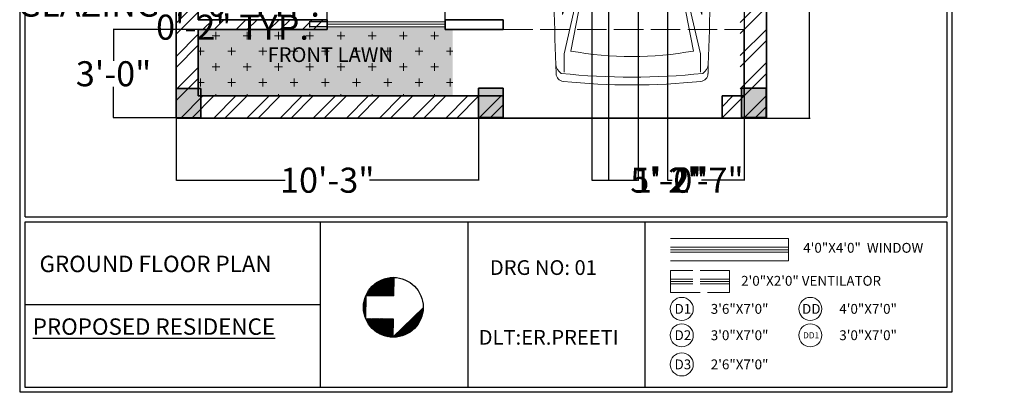
# Model space of a CAD drawing. Units: inches. Extents: x 1812 to 2791, y 2306 to 2959.
# Tile 1 of 8: x 1827 to 2227, y 2306 to 2458. Entities that reach past the tile are written whole.
import ezdxf

# ---------------------------------------------------------------- set-up
doc = ezdxf.new("R2010")
doc.units = ezdxf.units.IN
doc.linetypes.add('ACAD_ISO02W100', pattern=[15, 12, -3])
doc.layers.get('Defpoints').update_dxf_attribs({"lineweight": 50})
for name, color, linetype, lineweight in [('A-ANNO-DIMS', 2, 'Continuous', 18), ('A-ANNO-LEGD', 7, 'Continuous', 18), ('A-ANNO-SYMB', 7, 'Continuous', 18), ('A-ANNO-TEXT', 7, 'Continuous', 18), ('A-ANNO-TTLB', 7, 'Continuous', 25), ('A-AREA-IDEN', 7, 'Continuous', 18), ('A-COLS', 7, 'Continuous', 35), ('A-FURNITURE', 251, 'Continuous', 5), ('A-GLAZ-VENT', 6, 'ACAD_ISO02W100', 13), ('A-SITE-PARK', 8, 'Continuous', 13), ('A-WALL-OVHD', 30, 'ACAD_ISO02W100', 18), ('A-WALL-PATT', 8, 'Continuous', 13), ('L-PLNT-PATT', 8, 'Continuous', 13), ('WALL', 7, 'Continuous', 35), ('WINDOWS', 160, 'Continuous', 18)]:
    doc.layers.add(name, color=color, linetype=linetype, lineweight=lineweight)
doc.layers.add('L-PLNT-TURF-PATT', color=116, linetype='Continuous', lineweight=9, true_color=0x136734)
doc.layers.add('WALLS', color=7, linetype='Continuous')
doc.styles.add('1-100DIM', font='txt', dxfattribs={"height": 0.3})
doc.styles.get("Standard").update_dxf_attribs({"font": 'arial.ttf'})
doc.dimstyles.get("Standard").update_dxf_attribs({"dimtxt": 10.18, "dimasz": 0.18, "dimexe": 0.18, "dimexo": 0.0625, "dimgap": 0.09, "dimtad": 0, "dimtih": 1, "dimtoh": 1, "dimdec": 0, "dimzin": 0, "dimdsep": 46, "dimlunit": 3, "dimtxsty": 'Standard', "dimcen": 0.09, "dimadec": 0, "dimazin": 0, "dimtfac": 1, "dimtdec": 0, "dimtofl": 0, "dimtmove": 0, "dimatfit": 3, "dimfxl": 1, "dimtolj": 1, "dimtzin": 0, "dimarcsym": 0})

# ---------------------------------------------------------------- blocks, each defined once
blk = doc.blocks.new('CAR')
at = {"layer": 'A-FURNITURE'}
for p, q in [((2677.91, 1665.57), (2683.24, 1629.33)), ((2722.63, 1665.57), (2717.3, 1629.33)), ((2672.85, 1620.44), (2676.61, 1608)), ((2727.48, 1620.44), (2723.73, 1608)), ((2671.15, 1614.07), (2676.73, 1600.01)), ((2671.63, 1575.61), (2671.15, 1614.07)), ((2729.25, 1614.07), (2723.67, 1600.01)), ((2728.77, 1575.61), (2729.25, 1614.07)), ((2676.73, 1600.01), (2676.73, 1578.97)), ((2723.67, 1600.01), (2723.67, 1578.97)), ((2676.73, 1578.97), (2671.63, 1575.61)), ((2723.67, 1578.97), (2728.77, 1575.61)), ((2676.73, 1576.71), (2671.66, 1573.38)), ((2671.9, 1540.91), (2671.66, 1573.38)), ((2676.73, 1576.71), (2676.73, 1555.46)), ((2723.67, 1576.71), (2723.67, 1555.46)), ((2723.67, 1576.71), (2728.74, 1573.38)), ((2728.49, 1540.91), (2728.74, 1573.38)), ((2676.73, 1555.46), (2671.9, 1540.91)), ((2723.67, 1555.46), (2728.49, 1540.91)), ((2678.77, 1552.01), (2672.52, 1524.85)), ((2721.71, 1552.02), (2727.96, 1524.85)), ((2675.22, 1526.01), (2679.74, 1548.74)), ((2725.17, 1526.01), (2720.66, 1548.74)), ((2672.52, 1524.85), (2672.52, 1517.39)), ((2727.96, 1524.85), (2727.96, 1517.39))]:
    blk.add_line(p, q, dxfattribs=at)
for centre, radius, start, end in [((2699.3, 1570.19), 99.28, 73.0347, 105.8141), ((2699.3, 1552.83), 119.14, 76.3976, 102.667), ((2783.1, 1639.97), 115.47, 166.6607, 186.5655), ((2673.27, 1662.52), 3.34, 107.8179, 168.3942), ((2674, 1665.84), 3.34, 104.3452, 166.6607), ((2726.43, 1665.41), 3.34, 13.1156, 74.5941), ((2617.23, 1639.97), 115.47, 353.4345, 13.1156), ((2727.17, 1661.99), 3.34, 11.3249, 70.8826), ((4741.11, 1589.62), 2073.11, 178.89024, 182.01225), ((2700.17, 1579.09), 51.94, 60.0774, 119.9226), ((659.22, 1589.62), 2073.11, 357.98775, 1.10976), ((2675.91, 1621.37), 3.2, 121.1455, 196.7984), ((2724.42, 1621.37), 3.2, 343.2016, 58.8545), ((2679.67, 1608.92), 3.2, 196.7984, 283.6631), ((2700.17, 1519.83), 88.22, 77.0683, 102.9317), ((2720.66, 1608.92), 3.2, 256.3369, 343.2016), ((2700.16, 1829.45), 278.26, 265.5919, 274.4407), ((2700.17, 1827.63), 279.65, 265.7971, 274.2029), ((2700.17, 1663.47), 139.72, 259.6897, 280.3103), ((2674.03, 1521.04), 4.9, 184.3987, 237.5288), ((2726.3, 1521.04), 4.9, 302.4712, 355.6013), ((2672.62, 1516.95), 3.34, 182.1119, 263.4899), ((2700.17, 1791.26), 275.86, 264.0142, 275.9858), ((2700.17, 1790.18), 277.96, 264.2342, 275.7658), ((2727.71, 1516.95), 3.34, 276.5101, 357.8881)]:
    blk.add_arc(centre, radius, start, end, dxfattribs=at)
blk = doc.blocks.new('*D15')
at = {"layer": 'A-ANNO-DIMS', "color": 0, "lineweight": -2, "transparency": 16777216}
for p, q in [((2130.4, 2898), (2148.13, 2898)), ((2147.95, 2897.82), (2147.95, 2663.08)), ((2147.95, 2417.77), (2147.95, 2652.51)), ((2130.4, 2417.59), (2148.13, 2417.59))]:
    blk.add_line(p, q, dxfattribs=at)
at = {"layer": 'A-ANNO-DIMS', "color": 0, "transparency": 16777216}
for points in [[(2147.92, 2897.82), (2147.98, 2897.82), (2147.95, 2898)], [(2147.92, 2417.77), (2147.98, 2417.77), (2147.95, 2417.59)]]:
    blk.add_solid(points, dxfattribs=at)
at = {"layer": 'Defpoints', "color": 0, "transparency": 16777216}
for p in [(2130.34, 2898), (2130.34, 2417.59), (2147.95, 2417.59)]:
    blk.add_point(p, dxfattribs=at)
at = {"layer": 'A-ANNO-DIMS', "color": 0, "transparency": 16777216, "insert": (2147.95, 2657.8), "char_height": 10.18, "attachment_point": 5}
blk.add_mtext("\\A1;40'", dxfattribs=at)
blk = doc.blocks.new('COL')
at = {"transparency": 33554687}
h = blk.add_hatch(color=256, dxfattribs=at)
h.dxf.hatch_style = 1
h.paths.add_polyline_path([(2424.4, 2829.24), (2424.4, 2839.24), (2412.4, 2839.24), (2412.4, 2829.24)])
for p, q in [((2412.4, 2839.24), (2424.4, 2839.24)), ((2412.4, 2839.24), (2412.4, 2829.24)), ((2424.4, 2839.24), (2424.4, 2829.24)), ((2412.4, 2829.24), (2424.4, 2829.24))]:
    blk.add_line(p, q)
blk = doc.blocks.new('NORTH')
at = {"layer": 'WALLS'}
h = blk.add_hatch(dxfattribs=at)
h.set_pattern_fill('ANSI31', color=256, scale=6.087211)
h.set_pattern_definition([(45, (-41048.0969, 128612.4242), (-0.53803848, 0.53803848), [])])
h.paths.add_polyline_path([(6704.42, -25696.22), (6687.22, -25696.22, 0.302843), (6704.42, -25722.01)])
h.paths.add_polyline_path([(6743.1, -25696.22), (6725.9, -25696.22), (6725.9, -25722.01, 0.302843)])
h.paths.add_polyline_path([(6715.16, -25668.28), (6743.1, -25696.22, 0.414214)])
h.paths.add_polyline_path([(6725.9, -25722.01), (6704.42, -25722.01, 0.199872)])
for p, q in [((6743.1, -25696.22, 0.29), (6715.16, -25668.28, 0.29)), ((6687.22, -25696.22, 0.29), (6704.42, -25696.22, 0.29)), ((6704.42, -25722.01, 0.29), (6704.42, -25696.22, 0.29)), ((6725.9, -25722.01, 0.29), (6725.9, -25696.22, 0.29)), ((6725.9, -25696.22, 0.29), (6743.1, -25696.22, 0.29)), ((6704.42, -25722.01, 0.29), (6725.9, -25722.01, 0.29))]:
    blk.add_line(p, q, dxfattribs=at)
blk.add_circle((6715.16, -25696.22, 0.29), 27.94, dxfattribs=at)
blk = doc.blocks.new('VENT-24x9')
for p, q in [((3.5, 24), (3.5, 0)), ((4.5, 24), (4.5, 0)), ((5.5, 24), (5.5, 0))]:
    blk.add_line(p, q)
blk.add_lwpolyline([(0, 0), (9, 0), (9, 24), (0, 24)], close=True)
blk = doc.blocks.new('GLAZING-48x4')
for p, q in [((0, 2), (48, 2)), ((0, 1), (48, 1)), ((0, 0), (48, 0))]:
    blk.add_line(p, q)
blk = doc.blocks.new('WINDOW-LEGEND-48')
for p, q in [((48, 9), (0, 9)), ((48, 9), (48, 0)), ((48, 5.5), (0, 5.5)), ((48, 4.5), (0, 4.5)), ((48, 3.5), (0, 3.5)), ((0, 0), (48, 0))]:
    blk.add_line(p, q)
blk = doc.blocks.new('SHEET-FRAME-RESIDENCE')
for p, q in [((2, 71.32), (376.76, 71.32)), ((2, 69.32), (376.76, 69.32)), ((122.05, 1.92), (122.05, 69.32)), ((182.05, 1.92), (182.05, 69.32)), ((254.05, 1.92), (254.05, 69.32)), ((2, 35.72), (122.05, 35.72))]:
    blk.add_line(p, q)
blk.add_lwpolyline([(0, 632.8), (378.76, 632.8), (378.76, 0), (0, 0)], close=True)
for points in [[(2, 71.32), (2, 630.8), (376.76, 630.8), (376.76, 71.32)], [(376.76, 69.32), (376.76, 2), (2, 2), (2, 69.32)]]:
    blk.add_lwpolyline(points)
blk = doc.blocks.new('*D68')
at = {"layer": 'A-ANNO-DIMS', "color": 0, "lineweight": -2, "transparency": 16777216}
for p, q in [((1951.81, 2463.94), (1951.63, 2463.94)), ((1951.81, 2456.8), (1951.81, 2464.12)), ((1999.63, 2463.94), (1951.99, 2463.94)), ((1999.81, 2456.8), (1999.81, 2464.12))]:
    blk.add_line(p, q, dxfattribs=at)
at = {"layer": 'A-ANNO-DIMS', "color": 0, "transparency": 16777216}
for points in [[(1951.99, 2463.97), (1951.99, 2463.91), (1951.81, 2463.94)], [(1999.63, 2463.97), (1999.63, 2463.91), (1999.81, 2463.94)]]:
    blk.add_solid(points, dxfattribs=at)
at = {"layer": 'Defpoints', "color": 0, "transparency": 16777216}
for p in [(1951.81, 2463.94), (1951.81, 2456.74), (1999.81, 2456.74)]:
    blk.add_point(p, dxfattribs=at)
at = {"layer": 'A-ANNO-DIMS', "color": 0, "transparency": 16777216, "insert": (1887.41, 2463.94), "char_height": 10.18, "attachment_point": 5}
blk.add_mtext('\\A1;GLAZING 4\'-0" TYP.', dxfattribs=at)
blk = doc.blocks.new('*D69')
at = {"layer": 'A-ANNO-DIMS', "color": 0, "lineweight": -2, "transparency": 16777216}
for p, q in [((1951.75, 2456.74), (1944.43, 2456.74)), ((1951.75, 2454.74), (1944.43, 2454.74)), ((1944.61, 2454.56), (1944.43, 2454.56)), ((1944.61, 2456.56), (1944.61, 2454.92)), ((1944.61, 2454.74), (1944.61, 2454.56))]:
    blk.add_line(p, q, dxfattribs=at)
at = {"layer": 'A-ANNO-DIMS', "color": 0, "transparency": 16777216}
for points in [[(1944.58, 2456.56), (1944.64, 2456.56), (1944.61, 2456.74)], [(1944.58, 2454.92), (1944.64, 2454.92), (1944.61, 2454.74)]]:
    blk.add_solid(points, dxfattribs=at)
at = {"layer": 'Defpoints', "color": 0, "transparency": 16777216}
for p in [(1944.61, 2454.74), (1951.81, 2456.74), (1951.81, 2454.74)]:
    blk.add_point(p, dxfattribs=at)
at = {"layer": 'A-ANNO-DIMS', "color": 0, "transparency": 16777216, "insert": (1913.31, 2454.56), "char_height": 10.18, "attachment_point": 5}
blk.add_mtext('\\A1;0\'-2" TYP.', dxfattribs=at)
blk = doc.blocks.new('*D70')
at = {"layer": 'A-ANNO-DIMS', "color": 0, "lineweight": -2, "transparency": 16777216}
for p, q in [((1899.32, 2453.6), (1864.78, 2453.6)), ((1864.96, 2453.42), (1864.96, 2440.92)), ((1864.96, 2417.83), (1864.96, 2430.34)), ((1890.38, 2417.65), (1864.78, 2417.65))]:
    blk.add_line(p, q, dxfattribs=at)
at = {"layer": 'A-ANNO-DIMS', "color": 0, "transparency": 16777216}
for points in [[(1864.93, 2453.42), (1864.99, 2453.42), (1864.96, 2453.6)], [(1864.93, 2417.83), (1864.99, 2417.83), (1864.96, 2417.65)]]:
    blk.add_solid(points, dxfattribs=at)
at = {"layer": 'Defpoints', "color": 0, "transparency": 16777216}
for p in [(1864.96, 2453.6), (1899.39, 2453.6), (1890.44, 2417.65)]:
    blk.add_point(p, dxfattribs=at)
at = {"layer": 'A-ANNO-DIMS', "color": 0, "transparency": 16777216, "insert": (1864.96, 2435.63), "char_height": 10.18, "attachment_point": 5}
blk.add_mtext('\\A1;3\'-0"', dxfattribs=at)
blk = doc.blocks.new('*D71')
at = {"layer": 'A-ANNO-DIMS', "color": 0, "lineweight": -2, "transparency": 16777216}
for p, q in [((1890.39, 2417.54), (1890.39, 2392.17)), ((2013.32, 2417.72), (2013.32, 2392.17)), ((1890.57, 2392.35), (1934.76, 2392.35)), ((2013.14, 2392.35), (1968.95, 2392.35))]:
    blk.add_line(p, q, dxfattribs=at)
at = {"layer": 'A-ANNO-DIMS', "color": 0, "transparency": 16777216}
for points in [[(1890.57, 2392.38), (1890.57, 2392.32), (1890.39, 2392.35)], [(2013.14, 2392.38), (2013.14, 2392.32), (2013.32, 2392.35)]]:
    blk.add_solid(points, dxfattribs=at)
at = {"layer": 'Defpoints', "color": 0, "transparency": 16777216}
for p in [(1890.39, 2417.6), (2013.32, 2417.78), (2013.32, 2392.35)]:
    blk.add_point(p, dxfattribs=at)
at = {"layer": 'A-ANNO-DIMS', "color": 0, "transparency": 16777216, "insert": (1951.85, 2392.35), "char_height": 10.18, "attachment_point": 5}
blk.add_mtext('\\A1;10\'-3"', dxfattribs=at)
blk = doc.blocks.new('*D82')
at = {"layer": 'A-ANNO-DIMS', "color": 0, "lineweight": -2, "transparency": 16777216}
for p, q in [((2059.39, 2656.54), (2059.39, 2392.17)), ((2121.39, 2632.54), (2121.39, 2392.17)), ((2059.57, 2392.35), (2076.77, 2392.35)), ((2121.21, 2392.35), (2104.01, 2392.35))]:
    blk.add_line(p, q, dxfattribs=at)
at = {"layer": 'A-ANNO-DIMS', "color": 0, "transparency": 16777216}
for points in [[(2059.57, 2392.38), (2059.57, 2392.32), (2059.39, 2392.35)], [(2121.21, 2392.38), (2121.21, 2392.32), (2121.39, 2392.35)]]:
    blk.add_solid(points, dxfattribs=at)
at = {"layer": 'Defpoints', "color": 0, "transparency": 16777216}
for p in [(2059.39, 2656.6), (2121.39, 2632.6), (2121.39, 2392.35)]:
    blk.add_point(p, dxfattribs=at)
at = {"layer": 'A-ANNO-DIMS', "color": 0, "transparency": 16777216, "insert": (2090.39, 2392.35), "char_height": 10.18, "attachment_point": 5}
blk.add_mtext('\\A1;5\'-2"', dxfattribs=at)
blk = doc.blocks.new('*D86')
at = {"layer": 'A-ANNO-DIMS', "color": 0, "lineweight": -2, "transparency": 16777216}
for p, q in [((2066.19, 2594.54), (2066.19, 2392.17)), ((2078.19, 2594.54), (2078.19, 2392.17)), ((2066.37, 2392.35), (2078.01, 2392.35)), ((2078.19, 2392.35), (2078.37, 2392.35))]:
    blk.add_line(p, q, dxfattribs=at)
at = {"layer": 'A-ANNO-DIMS', "color": 0, "transparency": 16777216}
for points in [[(2066.37, 2392.38), (2066.37, 2392.32), (2066.19, 2392.35)], [(2078.01, 2392.38), (2078.01, 2392.32), (2078.19, 2392.35)]]:
    blk.add_solid(points, dxfattribs=at)
at = {"layer": 'Defpoints', "color": 0, "transparency": 16777216}
for p in [(2066.19, 2594.6), (2078.19, 2594.6), (2078.19, 2392.35)]:
    blk.add_point(p, dxfattribs=at)
at = {"layer": 'A-ANNO-DIMS', "color": 0, "transparency": 16777216, "insert": (2091.51, 2392.35), "char_height": 10.18, "attachment_point": 5}
blk.add_mtext('\\A1;1\'-0"', dxfattribs=at)
blk = doc.blocks.new('*D87')
at = {"layer": 'A-ANNO-DIMS', "color": 0, "lineweight": -2, "transparency": 16777216}
for p, q in [((2090.19, 2628.54), (2090.19, 2392.17)), ((2121.39, 2628.54), (2121.39, 2392.17)), ((2090.37, 2392.35), (2092.08, 2392.35)), ((2121.21, 2392.35), (2119.49, 2392.35))]:
    blk.add_line(p, q, dxfattribs=at)
at = {"layer": 'A-ANNO-DIMS', "color": 0, "transparency": 16777216}
for points in [[(2090.37, 2392.38), (2090.37, 2392.32), (2090.19, 2392.35)], [(2121.21, 2392.38), (2121.21, 2392.32), (2121.39, 2392.35)]]:
    blk.add_solid(points, dxfattribs=at)
at = {"layer": 'Defpoints', "color": 0, "transparency": 16777216}
for p in [(2090.19, 2628.6), (2121.39, 2628.6), (2121.39, 2392.35)]:
    blk.add_point(p, dxfattribs=at)
at = {"layer": 'A-ANNO-DIMS', "color": 0, "transparency": 16777216, "insert": (2105.79, 2392.35), "char_height": 10.18, "attachment_point": 5}
blk.add_mtext('\\A1;2\'-7"', dxfattribs=at)

msp = doc.modelspace()

# ---------------------------------------------------------------- hatches: boundary and pattern name
at = {"layer": 'A-WALL-PATT'}
h = msp.add_hatch(dxfattribs=at)
h.set_pattern_fill('ANSI32', color=256)
h.paths.add_polyline_path([(2130.39, 2417.6), (2119.69, 2417.6), (2119.69, 2768.56), (2121.39, 2768.56), (2121.39, 2801.62), (2121.32, 2849.36), (2121.32, 2801.62), (2130.39, 2801.62)])
h.paths.add_polyline_path([(2023.39, 2426.6), (1899.39, 2426.6), (1899.39, 2453.6), (1951.8, 2453.6), (1951.8, 2457.6), (1899.39, 2457.6), (1899.39, 2590.6), (1959.93, 2590.6), (1959.93, 2594.6), (1899.39, 2594.6), (1899.39, 2634.53), (1890.39, 2634.53), (1890.39, 2417.6), (2023.39, 2417.6)])
h.paths.add_polyline_path([(2119.69, 2426.6), (2112.39, 2426.6), (2112.39, 2417.6), (2119.69, 2417.6)])
h.paths.add_polyline_path([(1899.39, 2740.6), (1941.39, 2740.6), (1941.39, 2744.6), (1899.39, 2744.6), (1899.39, 2772.94), (1890.39, 2772.94), (1890.39, 2682.53), (1899.21, 2682.53), (1899.21, 2682.64)])
h.paths.add_polyline_path([(1975.39, 2838.6), (1899.39, 2838.6), (1899.39, 2856.33), (1890.39, 2856.33), (1890.39, 2796.95), (1899.39, 2796.95), (1899.39, 2834.6), (1971.39, 2834.6), (1971.39, 2740.6), (1975.39, 2740.6)])
h.paths.add_polyline_path([(2119.69, 2897.6), (1890.39, 2897.6), (1890.39, 2880.36), (1899.39, 2880.36), (1899.39, 2888.6), (2119.69, 2888.6)])
h.paths.add_polyline_path([(2130.39, 2897.6), (2119.69, 2897.6), (2119.69, 2888.6), (2121.39, 2888.6), (2121.39, 2849.62), (2130.39, 2849.62)])
at = {"layer": 'L-PLNT-PATT'}
h = msp.add_hatch(dxfattribs=at)
h.set_pattern_fill('CROSS', color=256)
h.paths.add_polyline_path([(2002.83, 2453.6), (1999.8, 2453.6), (1999.8, 2454.74), (1951.8, 2454.74), (1951.8, 2453.6), (1899.39, 2453.6), (1899.39, 2426.6), (2002.83, 2426.6)])
h.paths.add_polyline_path([(1925.4, 2437), (1983.81, 2437), (1983.81, 2449.37), (1925.4, 2449.37)], flags=24)
at = {"layer": 'L-PLNT-TURF-PATT', "transparency": 33554585}
h = msp.add_hatch(color=256, dxfattribs=at)
h.dxf.hatch_style = 1
h.paths.add_polyline_path([(2002.83, 2453.6), (1999.8, 2453.6), (1999.8, 2454.74), (1951.8, 2454.74), (1951.8, 2453.6), (1899.39, 2453.6), (1899.39, 2426.6), (2002.83, 2426.6)])
h.paths.add_polyline_path([(1925.4, 2437), (1983.81, 2437), (1983.81, 2449.37), (1925.4, 2449.37)], flags=24)

# ---------------------------------------------------------------- linework, layer by layer
at = {"layer": 'A-ANNO-LEGD'}
for centre in [(2095.98, 2340.03), (2148.23, 2340.03), (2095.98, 2329.31), (2148.23, 2329.31), (2095.98, 2317.46)]:
    msp.add_circle(centre, 4.67, dxfattribs=at)
at = {"layer": 'A-WALL-OVHD'}
msp.add_line((2023.39, 2453.6), (2121.39, 2453.6), dxfattribs=at)
at = {"layer": 'WALL'}
for p, q in [((2130.39, 2801.62), (2130.39, 2417.6)), ((1890.39, 2417.6), (1890.39, 2634.53)), ((1899.39, 2457.6), (1899.39, 2590.6)), ((1951.8, 2457.6), (1899.39, 2457.6)), ((1951.8, 2453.6), (1951.8, 2457.6)), ((2023.39, 2457.6), (1999.8, 2457.6)), ((1999.8, 2453.6), (1999.8, 2457.6)), ((2023.39, 2453.6), (2023.39, 2457.6)), ((1899.39, 2426.6), (1899.39, 2453.6)), ((1951.8, 2453.6), (1899.39, 2453.6)), ((2023.39, 2453.6), (1999.8, 2453.6)), ((2121.39, 2453.6), (2121.39, 2426.6)), ((2023.39, 2426.6), (1899.39, 2426.6)), ((2023.39, 2417.6), (2023.39, 2426.6)), ((2121.39, 2426.6), (2112.39, 2426.6)), ((2112.39, 2426.6), (2112.39, 2417.6)), ((2112.39, 2417.6), (1890.39, 2417.6)), ((2130.39, 2417.6), (2112.39, 2417.6))]:
    msp.add_line(p, q, dxfattribs=at)

# ---------------------------------------------------------------- block references
at = {"layer": 'A-ANNO-LEGD'}
msp.add_blockref('WINDOW-LEGEND-48', (2091.41, 2359.61), dxfattribs=at)
at = {"layer": 'A-ANNO-SYMB', "xscale": 0.4341621291417894, "yscale": 0.4341621291417894, "zscale": 0.4341621291417894, "rotation": 269.2509902977627}
msp.add_blockref('NORTH', (13172.19, 5110.05, -0.13), dxfattribs=at)
at = {"layer": 'A-ANNO-TTLB'}
msp.add_blockref('SHEET-FRAME-RESIDENCE', (1827.03, 2306.12), dxfattribs=at)
at = {"layer": 'A-COLS', "rotation": 270}
for p in [(-938.8, 4842.05), (-815.92, 4842.18), (-708.95, 4842.18)]:
    msp.add_blockref('COL', p, dxfattribs=at)
at = {"layer": 'A-GLAZ-VENT', "rotation": 270.0000000000015}
msp.add_blockref('VENT-24x9', (2091.41, 2355.66), dxfattribs=at)
at = {"layer": 'A-SITE-PARK'}
msp.add_blockref('CAR', (-624.41, 918.86), dxfattribs=at)
at = {"layer": 'WINDOWS', "rotation": 180}
msp.add_blockref('GLAZING-48x4', (1999.81, 2456.74), dxfattribs=at)

# ---------------------------------------------------------------- texts
at = {"layer": 'A-ANNO-TEXT', "attachment_point": 1}
for s, width, insert, char_height in [('4\'0"X4\'0"  WINDOW', 55.3456, (2145.35, 2366.86), 4), ('2\'0"X2\'0" VENTILATOR', 67.3186, (2120.1, 2353.44), 4), ('D1', 8.4888, (2093.04, 2342.04), 4), ('3\'6"X7\'0"', 8.4888, (2107.76, 2342.04), 4), ('DD', 8.4888, (2144.88, 2342.04), 4), ('4\'0"X7\'0"', 8.4888, (2160.01, 2342.04), 4), ('D2', 8.4888, (2093.04, 2331.33), 4), ('3\'0"X7\'0"', 8.4888, (2107.76, 2331.33), 4), ('DD1', 8.4888, (2145.29, 2330.55), 2.5), ('3\'0"X7\'0"', 8.4888, (2160.01, 2331.33), 4), ('D3', 8.4888, (2093.04, 2319.47), 4), ('2\'6"X7\'0"', 8.4888, (2107.76, 2319.47), 4)]:
    msp.add_mtext_dynamic_manual_height_columns(s, width=width, gutter_width=12.5, heights=[0], dxfattribs=dict(at, insert=insert, char_height=char_height))
at = {"layer": 'A-ANNO-TTLB', "char_height": 6.6726, "attachment_point": 1, "style": '1-100DIM'}
for s, width, insert in [('{\\f@Malgun Gothic|b0|i0|c0|p34;GROUND FLOOR PLAN }', 159.0041, (1834.85, 2361.66)), ('{\\f@Malgun Gothic|b0|i0|c0|p34;\\LPROPOSED RESIDENCE   }', 252.3616, (1832.1, 2336.17))]:
    msp.add_mtext_dynamic_manual_height_columns(s, width=width, gutter_width=13.96, heights=[0], dxfattribs=dict(at, insert=insert))
at = {"layer": 'A-ANNO-TTLB', "char_height": 6, "attachment_point": 1}
for s, insert in [('DRG NO: 01', (2017.97, 2359.84)), ('\\PDLT:ER.PREETI', (2013.41, 2341.47))]:
    msp.add_mtext_dynamic_manual_height_columns(s, width=58.1461, gutter_width=12.5, heights=[0], dxfattribs=dict(at, insert=insert))
at = {"layer": 'A-AREA-IDEN', "insert": (1927.59, 2446.38), "char_height": 6, "attachment_point": 1}
msp.add_mtext_dynamic_manual_height_columns('FRONT LAWN', width=184.4395, gutter_width=12.5, heights=[0], dxfattribs=at)

# ---------------------------------------------------------------- dimensions: what is measured, and where the dimension line sits
at = {"layer": 'A-ANNO-DIMS'}
dim = msp.add_linear_dim(base=(2147.95, 2417.59), p1=(2130.34, 2898), p2=(2130.34, 2417.59), angle=90, dimstyle='Standard', override={"dimclrd": 0, "dimclre": 0, "dimclrt": 0}, dxfattribs=at)
dim.commit()
dim.dimension.update_dxf_attribs({"geometry": '*D15', "text_midpoint": (2147.95, 2657.8), "dimtype": 160})
for base, p1, p2, picture, middle in [((2121.39, 2392.35), (2059.39, 2656.6), (2121.39, 2632.6), '*D82', (2090.39, 2392.35)), ((2121.39, 2392.35), (2090.19, 2628.6), (2121.39, 2628.6), '*D87', (2105.79, 2392.35)), ((2078.19, 2392.35), (2066.19, 2594.6), (2078.19, 2594.6), '*D86', (2091.51, 2392.35)), ((2013.32, 2392.35), (1890.39, 2417.6), (2013.32, 2417.78), '*D71', (1951.85, 2392.35))]:
    dim = msp.add_linear_dim(base=base, p1=p1, p2=p2, dimstyle='Standard', override={"dimdec": 1, "dimlfac": 1, "dimrnd": 0, "dimzin": 1, "dimdsep": 46, "dimlunit": 4, "dimfrac": 2}, dxfattribs=at)
    dim.commit()
    dim.dimension.update_dxf_attribs({"geometry": picture, "text_midpoint": middle})
for base, p1, p2, angle, text, picture, middle in [((1951.81, 2463.94), (1999.81, 2456.74), (1951.81, 2456.74), 180, 'GLAZING <> TYP.', '*D68', (1887.41, 2463.94)), ((1944.61, 2454.74), (1951.81, 2456.74), (1951.81, 2454.74), 270, '<> TYP.', '*D69', (1913.31, 2454.56))]:
    dim = msp.add_linear_dim(base=base, p1=p1, p2=p2, angle=angle, text=text, dimstyle='Standard', override={"dimdec": 1, "dimlfac": 1, "dimrnd": 0, "dimzin": 1, "dimdsep": 46, "dimlunit": 4, "dimfrac": 2}, dxfattribs=at)
    dim.commit()
    dim.dimension.update_dxf_attribs({"geometry": picture, "text_midpoint": middle})
dim = msp.add_linear_dim(base=(1864.9607, 2453.6029), p1=(1890.4404, 2417.6504), p2=(1899.3865, 2453.6029), angle=90, dimstyle='Standard', override={"dimdec": 1, "dimlfac": 1, "dimrnd": 0, "dimzin": 1, "dimdsep": 46, "dimlunit": 4, "dimfrac": 2}, dxfattribs=at)
dim.commit()
dim.dimension.update_dxf_attribs({"geometry": '*D70', "text_midpoint": (1864.9607, 2435.6267)})

doc.saveas('drawing.dxf')
